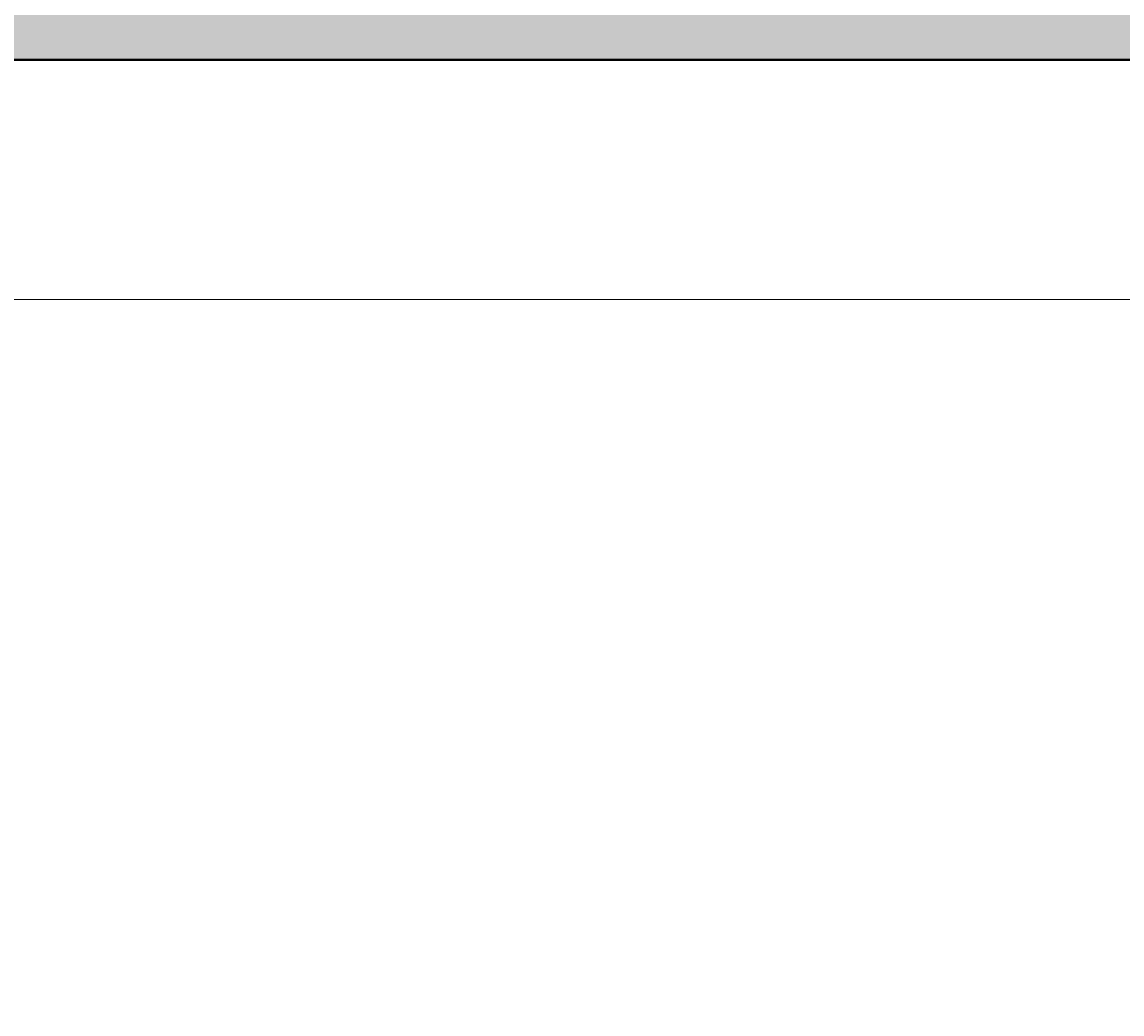
# Model space of a CAD drawing. Units: inches. Extents: x 1998 to 2588, y 1139 to 1977.
# Tile 86 of 134: x 2425 to 2453, y 1452 to 1477. Entities that reach past the tile are written whole.
import ezdxf

# ---------------------------------------------------------------- set-up
doc = ezdxf.new("R2010")
doc.units = ezdxf.units.IN
for name, color, linetype, lineweight in [('A-ANNO-DIMS', 2, 'Continuous', 18), ('A-WALL-PATT', 252, 'Continuous', 13), ('FUR', 21, 'Continuous', 18), ('WALL', 200, 'Continuous', 35)]:
    doc.layers.add(name, color=color, linetype=linetype, lineweight=lineweight)
doc.styles.get("Standard").update_dxf_attribs({"font": 'arial.ttf'})
doc.dimstyles.get("Standard").update_dxf_attribs({"dimtxt": 0.18, "dimasz": 0.18, "dimexe": 0.18, "dimexo": 0.0625, "dimgap": 0.09, "dimtad": 0, "dimtih": 1, "dimtoh": 1, "dimdec": 4, "dimzin": 0, "dimdsep": 46, "dimtxsty": 'Standard', "dimcen": 0.09, "dimadec": 0, "dimazin": 0, "dimtfac": 1, "dimtdec": 4, "dimtofl": 0, "dimtmove": 0, "dimatfit": 3, "dimfxl": 1, "dimtolj": 1, "dimtzin": 0, "dimarcsym": 0})

# ---------------------------------------------------------------- blocks, each defined once
blk = doc.blocks.new('CONSOLE-WALL')
blk.add_lwpolyline([(0, 6.123), (71.98, 6.123), (71.98, 0), (0, 0)], close=True)
blk = doc.blocks.new('*D23')
at = {"layer": 'A-ANNO-DIMS', "color": 0, "lineweight": -2, "transparency": 16777216}
for p, q in [((2549.179, 1476.17), (2549.179, 1138.602)), ((2059.473, 1413.17), (2059.473, 1138.602)), ((2059.653, 1138.782), (2303.928, 1138.782)), ((2548.999, 1138.782), (2304.723, 1138.782))]:
    blk.add_line(p, q, dxfattribs=at)
at = {"layer": 'A-ANNO-DIMS', "color": 0, "transparency": 16777216}
for points in [[(2059.653, 1138.812), (2059.653, 1138.752), (2059.473, 1138.782)], [(2548.999, 1138.812), (2548.999, 1138.752), (2549.179, 1138.782)]]:
    blk.add_solid(points, dxfattribs=at)
at = {"layer": 'Defpoints', "color": 0, "transparency": 16777216}
for p in [(2549.179, 1476.232), (2059.473, 1413.232), (2549.179, 1138.782)]:
    blk.add_point(p, dxfattribs=at)
at = {"layer": 'A-ANNO-DIMS', "color": 0, "transparency": 16777216, "insert": (2304.326, 1138.782), "char_height": 0.18, "attachment_point": 5}
blk.add_mtext('\\A1;489.7', dxfattribs=at)
blk = doc.blocks.new('*D24')
at = {"layer": 'A-ANNO-DIMS', "color": 0, "lineweight": -2, "transparency": 16777216}
for p, q in [((2398.535, 1911.232), (2588.309, 1911.232)), ((2588.129, 1911.052), (2588.129, 1570.164)), ((2588.129, 1228.912), (2588.129, 1569.8)), ((2527.535, 1228.732), (2588.309, 1228.732))]:
    blk.add_line(p, q, dxfattribs=at)
at = {"layer": 'A-ANNO-DIMS', "color": 0, "transparency": 16777216}
for points in [[(2588.099, 1911.052), (2588.159, 1911.052), (2588.129, 1911.232)], [(2588.099, 1228.912), (2588.159, 1228.912), (2588.129, 1228.732)]]:
    blk.add_solid(points, dxfattribs=at)
at = {"layer": 'Defpoints', "color": 0, "transparency": 16777216}
for p in [(2398.473, 1911.232), (2588.129, 1911.232), (2527.473, 1228.732)]:
    blk.add_point(p, dxfattribs=at)
at = {"layer": 'A-ANNO-DIMS', "color": 0, "transparency": 16777216, "insert": (2588.129, 1569.982), "char_height": 0.18, "attachment_point": 5}
blk.add_mtext('\\A1;682.5', dxfattribs=at)
blk = doc.blocks.new('*D33')
at = {"layer": 'A-ANNO-DIMS', "color": 0, "lineweight": -2, "transparency": 16777216}
for p, q in [((2407.973, 1480.67), (2407.973, 1138.602)), ((2498.179, 1480.67), (2498.179, 1138.602)), ((2408.153, 1138.782), (2452.753, 1138.782)), ((2497.999, 1138.782), (2453.399, 1138.782))]:
    blk.add_line(p, q, dxfattribs=at)
at = {"layer": 'A-ANNO-DIMS', "color": 0, "transparency": 16777216}
for points in [[(2408.153, 1138.812), (2408.153, 1138.752), (2407.973, 1138.782)], [(2497.999, 1138.812), (2497.999, 1138.752), (2498.179, 1138.782)]]:
    blk.add_solid(points, dxfattribs=at)
at = {"layer": 'Defpoints', "color": 0, "transparency": 16777216}
for p in [(2407.973, 1480.732), (2498.179, 1480.732), (2498.179, 1138.782)]:
    blk.add_point(p, dxfattribs=at)
at = {"layer": 'A-ANNO-DIMS', "color": 0, "transparency": 16777216, "insert": (2453.076, 1138.782), "char_height": 0.18, "attachment_point": 5}
blk.add_mtext('\\A1;90.2', dxfattribs=at)

msp = doc.modelspace()

# ---------------------------------------------------------------- hatches: boundary and pattern name
at = {"layer": 'A-WALL-PATT'}
h = msp.add_hatch(color=256, dxfattribs=at)
h.dxf.hatch_style = 1
h.paths.add_polyline_path([(2527.4729, 1362.2324), (2510.9729, 1362.2324), (2510.9729, 1357.7324), (2518.4729, 1357.7324), (2518.4729, 1237.7324), (2503.1458, 1237.7324), (2503.1458, 1228.7324), (2527.4729, 1228.7324)])
h.paths.add_polyline_path([(2490.5682, 1362.2324), (2398.4729, 1362.2324), (2398.4729, 1357.7324), (2490.5682, 1357.7324)])
h.paths.add_polyline_path([(2224.9729, 1264.7324), (2222.9729, 1264.7324), (2222.9729, 1232.4125), (2341.4729, 1232.4125), (2341.4729, 1234.4125), (2224.9729, 1234.4125)])
h.paths.add_polyline_path([(2334.5332, 1273.7324), (2264.7638, 1273.7324), (2264.7638, 1269.5611, -0.043659), (2264.3413, 1264.7324), (2334.5332, 1264.7324)])
h.paths.add_polyline_path([(2236.9551, 1273.7324), (2234.4125, 1273.7324), (2234.4125, 1264.7324), (2236.9551, 1264.7324), (2236.9551, 1269.5611)])
h.paths.add_polyline_path([(2222.9729, 1293.2324), (2096.9729, 1293.2324), (2096.9729, 1345.0966), (2087.9729, 1345.0966), (2087.9729, 1284.2324), (2222.9729, 1284.2324), (2222.9729, 1285.137)])
h.paths.add_polyline_path([(2096.9729, 1458.7927), (2087.9729, 1458.7927), (2087.9729, 1417.7324), (2087.9729, 1413.2324), (2096.9729, 1413.2324), (2096.9729, 1417.7324)])
h.paths.add_polyline_path([(2096.9729, 1413.2324), (2087.9729, 1413.2324), (2087.9729, 1365.5012), (2096.9729, 1365.5012), (2096.9729, 1369.3358)])
h.paths.add_polyline_path([(2186.2943, 1417.7324), (2138.6074, 1417.7324), (2096.9729, 1417.7324), (2096.9729, 1413.2324), (2138.6074, 1413.2324), (2186.2943, 1413.2324)])
h.paths.add_polyline_path([(2181.4729, 1465.7324), (2176.9729, 1465.7324), (2176.9729, 1451.6434), (2181.4729, 1451.6434)])
h.paths.add_polyline_path([(2181.4729, 1422.1664), (2176.9729, 1422.1664), (2176.9729, 1417.7324), (2181.4729, 1417.7324)])
h.paths.add_polyline_path([(2063.9729, 1465.7324), (2087.9729, 1465.7324), (2087.9729, 1470.2324), (2059.4729, 1470.2324), (2059.4729, 1413.2324), (2087.9729, 1413.2324), (2087.9729, 1417.7324), (2063.9729, 1417.7324)])
h.paths.add_polyline_path([(2181.4729, 1755.2324), (2176.9729, 1755.2324), (2176.9729, 1748.6798), (2177.0513, 1748.6798), (2181.4729, 1748.6798)])
h.paths.add_polyline_path([(2227.4729, 1707.2324), (2220.4647, 1707.2324), (2220.4647, 1702.7324), (2222.9729, 1702.7324), (2222.9729, 1604.637), (2227.4729, 1604.637)])
h.paths.add_polyline_path([(2114.9729, 1702.7324), (2105.9729, 1702.7324), (2105.9729, 1628.4781, -0.0318759), (2110.1012, 1628.7416), (2114.9729, 1628.7416)])
h.paths.add_polyline_path([(2345.9729, 1739.3278), (2341.4729, 1739.3278), (2341.4729, 1647.5211), (2345.9729, 1647.5211)])
h.paths.add_polyline_path([(2350.6273, 1641.2324), (2345.9729, 1641.2324), (2345.9729, 1636.7324), (2350.6273, 1636.7324), (2350.6273, 1639.8729)])
h.paths.add_polyline_path([(2501.9729, 1641.2324), (2407.9729, 1641.2324), (2392.5005, 1641.2324), (2392.5005, 1639.8729), (2392.5005, 1636.7324), (2501.9729, 1636.7324)])
h.paths.add_polyline_path([(2510.9729, 1755.2324), (2501.9729, 1755.2324), (2501.9729, 1641.2324), (2510.9729, 1641.2324)])
h.paths.add_polyline_path([(2549.1786, 1641.2324), (2522.3775, 1641.2324), (2522.3775, 1636.7324), (2540.1786, 1636.7324), (2540.1786, 1480.7324), (2522.3775, 1480.7324), (2522.3775, 1476.2324), (2549.1786, 1476.2324)])
h.paths.add_polyline_path([(2498.1786, 1594.7324), (2407.9729, 1594.7324), (2407.9729, 1585.7324), (2416.9729, 1585.7324), (2489.1786, 1585.7324), (2489.1786, 1531.7324), (2416.9729, 1531.7324), (2407.9729, 1531.7324), (2407.9729, 1522.7324), (2498.1786, 1522.7324)])
h.paths.add_polyline_path([(2351.6437, 1480.7324), (2345.9729, 1480.7324), (2345.9729, 1476.2324), (2351.6437, 1476.2324), (2351.6437, 1477.5919)])
h.paths.add_polyline_path([(2501.9729, 1480.7324), (2498.1786, 1480.7324), (2407.9729, 1480.7324), (2393.5168, 1480.7324), (2393.5168, 1477.5919), (2393.5168, 1476.2324), (2501.9729, 1476.2324)])

# ---------------------------------------------------------------- linework, layer by layer
at = {"layer": 'WALL'}
for p, q in [((2392.6008, 1476.2324), (2501.9729, 1476.2324)), ((2501.9729, 1476.2324), (2407.9729, 1476.2324))]:
    msp.add_line(p, q, dxfattribs=at)

# ---------------------------------------------------------------- block references
at = {"layer": 'FUR'}
msp.add_blockref('CONSOLE-WALL', (2415.1012, 1470.109), dxfattribs=at)

# ---------------------------------------------------------------- dimensions: what is measured, and where the dimension line sits
at = {"layer": 'A-ANNO-DIMS'}
dim = msp.add_linear_dim(base=(2588.1286, 1911.2324), p1=(2527.4729, 1228.7324), p2=(2398.4729, 1911.2324), angle=90, dimstyle='Standard', override={"dimdec": 1, "dimlfac": 1, "dimrnd": 0, "dimzin": 0, "dimdsep": 46, "dimlunit": 2}, dxfattribs=at)
dim.commit()
dim.dimension.update_dxf_attribs({"geometry": '*D24', "text_midpoint": (2588.1286, 1569.9824)})
for base, p1, p2, picture, middle in [((2498.1786, 1138.7824), (2407.9729, 1480.7324), (2498.1786, 1480.7324), '*D33', (2453.0757, 1138.7824)), ((2549.1786, 1138.7824), (2059.4729, 1413.2324), (2549.1786, 1476.2324), '*D23', (2304.3257, 1138.7824))]:
    dim = msp.add_linear_dim(base=base, p1=p1, p2=p2, dimstyle='Standard', override={"dimdec": 1, "dimlfac": 1, "dimrnd": 0, "dimzin": 0, "dimdsep": 46, "dimlunit": 2}, dxfattribs=at)
    dim.commit()
    dim.dimension.update_dxf_attribs({"geometry": picture, "text_midpoint": middle})

doc.saveas('drawing.dxf')
